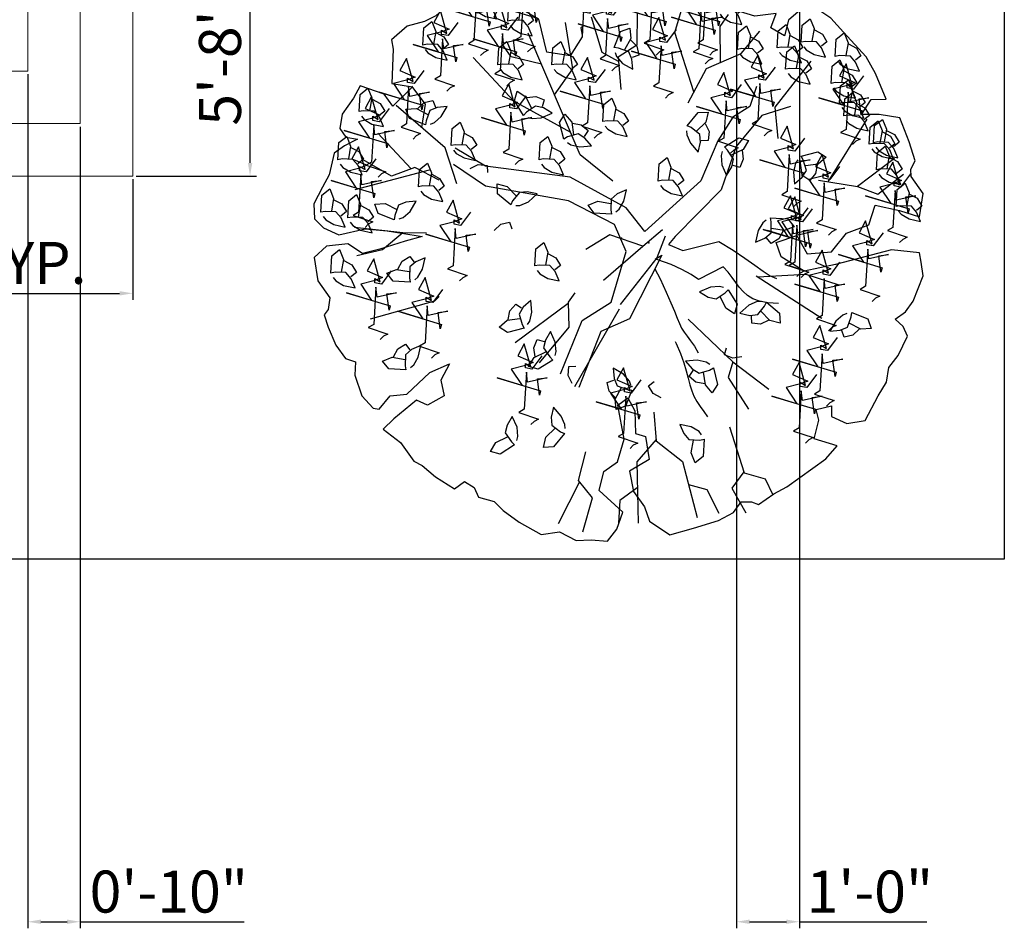
# Model space of a CAD drawing. Units: inches. Extents: x 3394 to 4794, y 965 to 1718.
# Tile 2 of 15: x 3753 to 3941, y 987 to 1160. Entities that reach past the tile are written whole.
import ezdxf

# ---------------------------------------------------------------- set-up
doc = ezdxf.new("R2010")
doc.units = ezdxf.units.IN
for name, color, linetype, lineweight in [('A-ANNO-DIMS', 2, 'Continuous', 13), ('A-FLOR-STRS', 7, 'Continuous', 18), ('C-PROP', 7, 'Continuous', 25), ('CAY', 94, 'Continuous', 13)]:
    doc.layers.add(name, color=color, linetype=linetype, lineweight=lineweight)
doc.layers.add('ARBOL', color=74, linetype='Continuous')
doc.layers.add('TALLO', color=36, linetype='Continuous')
doc.styles.get("Standard").update_dxf_attribs({"font": 'arial.ttf'})
doc.dimstyles.new('ISO-25', dxfattribs={"dimtxt": 8, "dimasz": 2.5, "dimexe": 1.25, "dimexo": 0.625, "dimtad": 1, "dimlunit": 3, "dimtxsty": 'Standard', "dimcen": 2.5, "dimadec": 0, "dimazin": 0, "dimtfac": 1, "dimtmove": 0, "dimatfit": 3, "dimfxl": 1, "dimarcsym": 0})

# ---------------------------------------------------------------- blocks, each defined once
blk = doc.blocks.new('fresno')
at = {"layer": 'ARBOL'}
for p, q in [((2.96, 0.991), (3.575, 1.984)), ((-3.638, 1.194), (-4.164, 1.76)), ((-1.151, -0.932), (-1.99, -1.556)), ((-0.974, -3.757), (-1.31, -4.423))]:
    blk.add_line(p, q, dxfattribs=at)
blk.add_lwpolyline([(0.823, 4.745), (0.566, 4.764), (0.459, 4.687), (0.336, 4.518), (0.233, 4.322), (0.087, 4.298), (0.091, 4.464), (0.14, 4.621), (-0.09, 4.659), (-0.033, 4.863), (-0.264, 4.901), (-0.483, 4.866), (-0.686, 4.924), (-1.021, 4.801), (-1.288, 4.8), (-1.431, 4.563), (-1.234, 4.327), (-1.406, 4), (-1.205, 3.778), (-0.909, 3.705), (-0.931, 3.283), (-1.122, 2.983), (-1.491, 3.043), (-1.619, 3.562), (-1.9, 3.727), (-1.851, 3.982), (-2.197, 4.084), (-2.278, 4.31), (-2.543, 4.283), (-2.896, 4.152), (-3.091, 3.971), (-3.022, 3.817), (-3.244, 3.617), (-3.424, 3.528), (-3.697, 3.455), (-3.946, 3.236), (-3.922, 3.09), (-3.94, 2.548), (-3.617, 2.495), (-3.927, 2.19), (-4.062, 2.379), (-4.443, 2.512), (-4.546, 2.316), (-4.73, 2.062), (-4.767, 1.832), (-4.671, 1.698), (-4.486, 1.667), (-4.693, 1.559), (-4.854, 1.444), (-4.934, 1.102), (-5.037, 0.905), (-5.175, 0.644), (-5.166, 0.406), (-5.024, 0.264), (-4.781, 0.153), (-4.363, 0.249), (-4.014, 0.215), (-3.783, 0.177), (-3.46, 0.124), (-3.733, 0.051), (-4.132, -0.073), (-4.404, -0.146), (-4.639, 0.011), (-4.977, -0.028), (-5.172, -0.209), (-5.113, -0.574), (-4.921, -0.843), (-4.951, -1.027), (-5.012, -1.112), (-4.95, -1.311), (-4.83, -1.592), (-4.676, -1.807), (-4.518, -1.856), (-4.529, -2.068), (-4.417, -2.394), (-4.236, -2.59), (-4.143, -2.605), (-3.967, -2.397), (-3.703, -2.37), (-3.339, -2.027), (-3.032, -1.889), (-3.169, -2.15), (-3.115, -2.396), (-3.376, -2.542), (-3.552, -2.466), (-3.909, -2.762), (-4.077, -2.924), (-3.804, -3.135), (-3.592, -3.43), (-3.461, -3.499), (-3.253, -3.676), (-2.953, -3.867), (-2.792, -3.752), (-2.642, -3.848), (-2.572, -4.001), (-2.323, -4.066), (-2.18, -4.208), (-1.926, -4.392), (-1.58, -4.591), (-1.288, -4.545), (-1.027, -4.683), (-0.788, -4.675), (-0.531, -4.693), (-0.382, -4.505), (-0.29, -4.236), (-0.66, -3.891), (-0.588, -3.595), (-0.374, -3.441), (-0.267, -3.079), (-0.368, -2.541), (-0.208, -2.426), (-0.099, -2.633), (-0.087, -2.991), (0.071, -3.04), (0.129, -3.405), (-0.185, -3.59), (-0.119, -3.909), (0.055, -4.151), (0.136, -4.377), (0.456, -4.596), (0.828, -4.491), (1.227, -4.368), (1.461, -4.241), (1.583, -4.071), (1.748, -4.075), (1.86, -4.117), (2.101, -3.944), (2.308, -3.836), (2.925, -3.393), (3.101, -3.185), (2.74, -3.078), (2.812, -2.782), (2.769, -2.61), (3.015, -2.555), (3.012, -2.721), (3.254, -2.832), (3.546, -2.785), (3.752, -2.393), (3.882, -2.177), (3.92, -1.947), (4.069, -1.758), (4.214, -1.451), (4.144, -1.297), (4.021, -1.182), (4.182, -1.067), (4.304, -0.897), (4.464, -0.497), (4.429, -0.279), (4.406, -0.133), (3.964, -0.083), (3.074, -0.315), (2.582, -0.424), (2.217, -0.197), (2.136, 0.029), (2.462, 0.141), (2.628, -0.147), (3.012, -0.116), (3.249, 0.177), (3.602, 0.308), (3.701, 0.623), (4.089, 0.535), (4.404, 0.436), (4.464, 0.805), (4.272, 1.074), (4.267, 1.193), (4.336, 1.324), (4.243, 1.623), (4.092, 2.003), (3.769, 2.057), (3.485, 2.056), (3.642, 2.291), (3.88, 2.299), (3.71, 2.706), (3.563, 2.967), (3.201, 3.358), (3.001, 3.581), (2.766, 3.738), (2.635, 3.807), (2.332, 3.549), (2.268, 3.299), (2.052, 3.429), (2.136, 3.652), (1.798, 3.613), (1.437, 3.72), (1.755, 4.071), (1.513, 4.182), (1.451, 4.381), (1.519, 4.512), (1.204, 4.611), (1.012, 4.596)], close=True, dxfattribs=at)
for points in [[(-1.104, 4.45), (-1.063, 4.399), (-0.939, 4.325), (-0.757, 4.285), (-0.82, 4.431), (-0.903, 4.527), (-1.075, 4.533), (-1.143, 4.521), (-1.126, 4.792), (-1.002, 4.891), (-0.939, 4.738), (-0.975, 4.535)], [(-0.346, 4.735), (-0.501, 4.528), (-0.605, 4.545), (-0.605, 4.614), (-0.519, 4.563), (-0.622, 4.925), (-0.726, 4.735), (-0.484, 4.632), (-0.622, 4.58), (-0.829, 4.528), (-0.657, 4.27), (-1.053, 4.39), (-0.363, 4.183), (-0.381, 4.114), (-0.415, 4.373), (-0.26, 4.39), (-0.57, 4.321), (-0.588, 4.476), (-0.622, 3.89), (-0.708, 3.839), (-0.398, 3.735), (-0.467, 3.701), (-0.519, 3.649)], [(-0.935, 4.717), (-0.809, 4.65), (-0.736, 4.529), (-0.824, 4.459)], [(0.263, 4.114), (0.304, 4.063), (0.429, 3.989), (0.611, 3.948), (0.547, 4.095), (0.465, 4.191), (0.293, 4.197), (0.225, 4.185), (0.242, 4.456), (0.366, 4.555), (0.428, 4.402), (0.393, 4.199)], [(0.734, 4.203), (0.775, 4.152), (0.9, 4.078), (1.082, 4.038), (1.018, 4.185), (0.936, 4.281), (0.763, 4.287), (0.696, 4.274), (0.712, 4.546), (0.837, 4.645), (0.899, 4.491), (0.863, 4.289)], [(-0.521, 4.069), (-0.48, 4.018), (-0.356, 3.944), (-0.174, 3.904), (-0.237, 4.051), (-0.32, 4.146), (-0.492, 4.152), (-0.56, 4.14), (-0.543, 4.411), (-0.419, 4.511), (-0.356, 4.357), (-0.392, 4.154)], [(0.433, 4.381), (0.558, 4.314), (0.631, 4.193), (0.544, 4.122)], [(0.904, 4.471), (1.029, 4.404), (1.102, 4.282), (1.015, 4.212)], [(-2.368, 4.073), (-2.523, 3.866), (-2.627, 3.883), (-2.627, 3.952), (-2.541, 3.9), (-2.644, 4.262), (-2.748, 4.073), (-2.506, 3.969), (-2.644, 3.918), (-2.851, 3.866), (-2.679, 3.607), (-3.075, 3.728), (-2.385, 3.521), (-2.403, 3.452), (-2.437, 3.711), (-2.282, 3.728), (-2.592, 3.659), (-2.61, 3.814), (-2.644, 3.228), (-2.73, 3.176), (-2.42, 3.073), (-2.489, 3.038), (-2.541, 2.987)], [(-1.623, 4.132), (-1.778, 3.925), (-1.882, 3.942), (-1.882, 4.011), (-1.795, 3.959), (-1.899, 4.321), (-2.002, 4.132), (-1.761, 4.028), (-1.899, 3.977), (-2.106, 3.925), (-1.933, 3.666), (-2.33, 3.787), (-1.64, 3.58), (-1.657, 3.511), (-1.692, 3.77), (-1.537, 3.787), (-1.847, 3.718), (-1.864, 3.873), (-1.899, 3.287), (-1.985, 3.235), (-1.675, 3.132), (-1.744, 3.097), (-1.795, 3.046)], [(-1.149, 3.822), (-1.108, 3.771), (-0.983, 3.697), (-0.802, 3.657), (-0.865, 3.804), (-0.948, 3.9), (-1.12, 3.906), (-1.188, 3.893), (-1.171, 4.165), (-1.047, 4.264), (-0.984, 4.111), (-1.02, 3.908)], [(-0.352, 4.337), (-0.226, 4.269), (-0.153, 4.148), (-0.241, 4.078)], [(0.413, 4.08), (0.258, 3.873), (0.154, 3.89), (0.154, 3.959), (0.241, 3.908), (0.137, 4.27), (0.034, 4.08), (0.275, 3.977), (0.137, 3.925), (-0.07, 3.873), (0.103, 3.614), (-0.294, 3.735), (0.396, 3.528), (0.379, 3.459), (0.344, 3.718), (0.499, 3.735), (0.189, 3.666), (0.172, 3.821), (0.137, 3.235), (0.051, 3.183), (0.361, 3.08), (0.292, 3.046), (0.241, 2.994)], [(1.259, 4.08), (1.103, 3.873), (1, 3.89), (1, 3.959), (1.086, 3.908), (0.982, 4.27), (0.879, 4.08), (1.12, 3.977), (0.982, 3.925), (0.775, 3.873), (0.948, 3.614), (0.551, 3.735), (1.241, 3.528), (1.224, 3.459), (1.189, 3.718), (1.345, 3.735), (1.034, 3.666), (1.017, 3.821), (0.982, 3.235), (0.896, 3.183), (1.207, 3.08), (1.138, 3.046), (1.086, 2.994)], [(-2.629, 3.733), (-2.588, 3.682), (-2.463, 3.608), (-2.281, 3.568), (-2.345, 3.715), (-2.427, 3.81), (-2.6, 3.816), (-2.667, 3.804), (-2.651, 4.075), (-2.526, 4.175), (-2.464, 4.021), (-2.5, 3.818)], [(-0.98, 4.09), (-0.854, 4.023), (-0.781, 3.901), (-0.869, 3.831)], [(1.189, 3.942), (1.034, 3.735), (0.931, 3.752), (0.931, 3.821), (1.017, 3.77), (0.913, 4.132), (0.81, 3.942), (1.051, 3.839), (0.913, 3.787), (0.706, 3.735), (0.879, 3.477), (0.482, 3.597), (1.172, 3.39), (1.155, 3.321), (1.12, 3.58), (1.276, 3.597), (0.965, 3.528), (0.948, 3.683), (0.913, 3.097), (0.827, 3.046), (1.138, 2.942), (1.069, 2.908), (1.017, 2.856)], [(1.25, 3.643), (1.291, 3.592), (1.416, 3.518), (1.597, 3.478), (1.534, 3.625), (1.451, 3.721), (1.279, 3.727), (1.211, 3.714), (1.228, 3.985), (1.352, 4.085), (1.415, 3.931), (1.379, 3.729)], [(-2.459, 4), (-2.334, 3.933), (-2.261, 3.812), (-2.348, 3.742)], [(-2.068, 3.464), (-2.027, 3.413), (-1.903, 3.339), (-1.721, 3.299), (-1.784, 3.446), (-1.867, 3.542), (-2.039, 3.547), (-2.107, 3.535), (-2.09, 3.806), (-1.966, 3.906), (-1.903, 3.752), (-1.939, 3.55)], [(-0.287, 3.833), (-0.442, 3.626), (-0.546, 3.643), (-0.546, 3.712), (-0.46, 3.661), (-0.563, 4.023), (-0.667, 3.833), (-0.425, 3.73), (-0.563, 3.678), (-0.77, 3.626), (-0.598, 3.367), (-0.995, 3.488), (-0.304, 3.281), (-0.322, 3.212), (-0.356, 3.471), (-0.201, 3.488), (-0.511, 3.419), (-0.529, 3.574), (-0.563, 2.988), (-0.649, 2.936), (-0.339, 2.833), (-0.408, 2.799), (-0.46, 2.747)], [(0.837, 2.414), (0.533, 3.352), (0.697, 3.906)], [(1.419, 3.911), (1.545, 3.844), (1.618, 3.722), (1.53, 3.652)], [(-1.951, 3.597), (-2.106, 3.39), (-2.209, 3.408), (-2.209, 3.477), (-2.123, 3.425), (-2.227, 3.787), (-2.33, 3.597), (-2.089, 3.494), (-2.227, 3.442), (-2.434, 3.39), (-2.261, 3.132), (-2.658, 3.252), (-1.968, 3.046), (-1.985, 2.977), (-2.02, 3.235), (-1.864, 3.252), (-2.175, 3.183), (-2.192, 3.339), (-2.227, 2.752), (-2.313, 2.701), (-2.002, 2.597), (-2.071, 2.563), (-2.123, 2.511)], [(-2.898, 3.511), (-3.053, 3.304), (-3.157, 3.321), (-3.157, 3.39), (-3.071, 3.339), (-3.174, 3.701), (-3.278, 3.511), (-3.036, 3.408), (-3.174, 3.356), (-3.381, 3.304), (-3.209, 3.046), (-3.605, 3.166), (-2.915, 2.959), (-2.932, 2.89), (-2.967, 3.149), (-2.812, 3.166), (-3.122, 3.097), (-3.14, 3.253), (-3.174, 2.666), (-3.26, 2.615), (-2.95, 2.511), (-3.019, 2.477), (-3.071, 2.425)], [(-1.899, 3.732), (-1.773, 3.664), (-1.7, 3.543), (-1.788, 3.473)], [(-0.358, 2.895), (-0.615, 3.037), (-0.783, 3.596)], [(-0.063, 3.671), (-0.069, 3.151), (-0.364, 2.965), (-0.319, 2.449)], [(0.558, 3.402), (0.403, 3.195), (0.299, 3.212), (0.299, 3.281), (0.386, 3.23), (0.282, 3.592), (0.179, 3.402), (0.42, 3.299), (0.282, 3.247), (0.075, 3.195), (0.248, 2.936), (-0.149, 3.057), (0.541, 2.85), (0.524, 2.781), (0.489, 3.04), (0.644, 3.057), (0.334, 2.988), (0.317, 3.143), (0.282, 2.557), (0.196, 2.505), (0.506, 2.402), (0.437, 2.368), (0.386, 2.316)], [(1.259, 2.882), (1.254, 3.446), (1.381, 3.636)], [(-3.413, 3.083), (-3.373, 3.032), (-3.248, 2.958), (-3.066, 2.918), (-3.129, 3.065), (-3.212, 3.161), (-3.384, 3.167), (-3.452, 3.154), (-3.435, 3.425), (-3.311, 3.525), (-3.248, 3.371), (-3.284, 3.169)], [(-1.367, 2.367), (-1.081, 2.78), (-1.193, 3.514)], [(-0.923, 3.449), (-0.951, 3.425), (-0.93, 3.313)], [(1.564, 3.016), (1.605, 2.965), (1.729, 2.891), (1.911, 2.851), (1.848, 2.998), (1.765, 3.094), (1.593, 3.099), (1.525, 3.087), (1.542, 3.358), (1.666, 3.458), (1.729, 3.304), (1.693, 3.102)], [(2.191, 3.038), (2.232, 2.987), (2.357, 2.913), (2.539, 2.873), (2.475, 3.02), (2.393, 3.116), (2.221, 3.122), (2.153, 3.109), (2.17, 3.381), (2.294, 3.48), (2.356, 3.326), (2.321, 3.124)], [(2.573, 3.128), (2.613, 3.077), (2.738, 3.003), (2.92, 2.963), (2.857, 3.11), (2.774, 3.205), (2.602, 3.211), (2.534, 3.199), (2.551, 3.47), (2.675, 3.57), (2.738, 3.416), (2.702, 3.214)], [(-3.244, 3.351), (-3.118, 3.284), (-3.045, 3.162), (-3.133, 3.092)], [(-0.448, 1), (-0.961, 1.419), (-1.784, 3.341)], [(-0.41, 3.035), (-0.387, 2.974), (-0.291, 2.865), (-0.131, 2.771), (-0.146, 2.93), (-0.195, 3.047), (-0.357, 3.106), (-0.425, 3.115), (-0.325, 3.368), (-0.176, 3.424), (-0.164, 3.258), (-0.261, 3.077)], [(0.746, 2.242), (1.034, 2.786), (1.584, 3.019), (1.879, 3.374)], [(1.733, 3.284), (1.859, 3.216), (1.932, 3.095), (1.844, 3.025)], [(2.361, 3.306), (2.486, 3.239), (2.559, 3.117), (2.472, 3.047)], [(2.742, 3.396), (2.868, 3.328), (2.941, 3.207), (2.853, 3.137)], [(3.111, 2.904), (3.152, 2.853), (3.276, 2.779), (3.458, 2.739), (3.395, 2.886), (3.312, 2.981), (3.14, 2.987), (3.072, 2.975), (3.089, 3.246), (3.213, 3.346), (3.276, 3.192), (3.24, 2.99)], [(-2.225, 2.77), (-2.184, 2.718), (-2.06, 2.645), (-1.878, 2.604), (-1.941, 2.751), (-2.024, 2.847), (-2.196, 2.853), (-2.264, 2.84), (-2.247, 3.112), (-2.123, 3.211), (-2.06, 3.058), (-2.096, 2.855)], [(-1.575, 2.854), (-2.052, 2.969), (-2.2, 3.178)], [(-1.373, 2.77), (-1.332, 2.718), (-1.208, 2.645), (-1.026, 2.604), (-1.089, 2.751), (-1.172, 2.847), (-1.344, 2.853), (-1.412, 2.84), (-1.395, 3.112), (-1.271, 3.211), (-1.208, 3.058), (-1.244, 2.855)], [(-0.166, 3.238), (-0.068, 3.135), (-0.036, 2.997), (-0.141, 2.957)], [(2.326, 2.702), (2.367, 2.651), (2.492, 2.577), (2.673, 2.537), (2.61, 2.684), (2.527, 2.78), (2.355, 2.786), (2.287, 2.773), (2.304, 3.045), (2.428, 3.144), (2.491, 2.99), (2.455, 2.788)], [(3.28, 3.172), (3.406, 3.104), (3.479, 2.983), (3.391, 2.913)], [(-2.056, 3.037), (-1.93, 2.97), (-1.857, 2.849), (-1.945, 2.778)], [(-0.57, 2.77), (-0.726, 2.563), (-0.829, 2.58), (-0.829, 2.649), (-0.743, 2.597), (-0.846, 2.959), (-0.95, 2.77), (-0.708, 2.666), (-0.846, 2.615), (-1.053, 2.563), (-0.881, 2.304), (-1.278, 2.425), (-0.588, 2.218), (-0.605, 2.149), (-0.639, 2.408), (-0.484, 2.425), (-0.795, 2.356), (-0.812, 2.511), (-0.846, 1.925), (-0.933, 1.873), (-0.622, 1.77), (-0.691, 1.735), (-0.743, 1.684)], [(-1.204, 3.037), (-1.078, 2.97), (-1.005, 2.849), (-1.093, 2.778)], [(2.121, 2.804), (1.966, 2.597), (1.862, 2.615), (1.862, 2.683), (1.949, 2.632), (1.845, 2.994), (1.742, 2.804), (1.983, 2.701), (1.845, 2.649), (1.638, 2.597), (1.811, 2.339), (1.414, 2.459), (2.104, 2.252), (2.087, 2.184), (2.052, 2.442), (2.207, 2.459), (1.897, 2.39), (1.88, 2.546), (1.845, 1.959), (1.759, 1.908), (2.069, 1.804), (2, 1.77), (1.949, 1.718)], [(2.495, 2.97), (2.621, 2.903), (2.694, 2.781), (2.606, 2.711)], [(-3.434, 2.752), (-3.59, 2.546), (-3.693, 2.563), (-3.693, 2.632), (-3.607, 2.58), (-3.71, 2.942), (-3.814, 2.752), (-3.572, 2.649), (-3.71, 2.597), (-3.917, 2.546), (-3.745, 2.287), (-4.142, 2.408), (-3.452, 2.201), (-3.469, 2.132), (-3.503, 2.39), (-3.348, 2.408), (-3.659, 2.339), (-3.676, 2.494), (-3.71, 1.908), (-3.797, 1.856), (-3.486, 1.753), (-3.555, 1.718), (-3.607, 1.666)], [(-1.112, 1.773), (-2.014, 2.265), (-2.654, 2.957)], [(2.171, 1.674), (2.121, 2.172), (2.689, 2.898)], [(3.519, 2.666), (3.363, 2.459), (3.26, 2.477), (3.26, 2.546), (3.346, 2.494), (3.243, 2.856), (3.139, 2.666), (3.381, 2.563), (3.243, 2.511), (3.036, 2.459), (3.208, 2.201), (2.811, 2.321), (3.501, 2.115), (3.484, 2.046), (3.45, 2.304), (3.605, 2.321), (3.294, 2.252), (3.277, 2.408), (3.243, 1.821), (3.156, 1.77), (3.467, 1.666), (3.398, 1.632), (3.346, 1.58)], [(3.043, 2.478), (3.084, 2.427), (3.209, 2.353), (3.391, 2.313), (3.327, 2.46), (3.245, 2.556), (3.073, 2.562), (3.005, 2.549), (3.022, 2.82), (3.146, 2.92), (3.208, 2.766), (3.173, 2.564)], [(1.586, 2.528), (1.431, 2.321), (1.327, 2.339), (1.327, 2.408), (1.414, 2.356), (1.31, 2.718), (1.207, 2.528), (1.448, 2.425), (1.31, 2.373), (1.103, 2.321), (1.276, 2.063), (0.879, 2.184), (1.569, 1.977), (1.552, 1.908), (1.517, 2.166), (1.673, 2.184), (1.362, 2.115), (1.345, 2.27), (1.31, 1.684), (1.224, 1.632), (1.535, 1.528), (1.466, 1.494), (1.414, 1.442)], [(3.213, 2.746), (3.338, 2.679), (3.411, 2.557), (3.324, 2.487)], [(-3.468, 1.85), (-3.409, 2.222), (-3.628, 2.505)], [(-1.817, 2.351), (-1.972, 2.144), (-2.075, 2.162), (-2.075, 2.231), (-1.989, 2.179), (-2.093, 2.541), (-2.196, 2.351), (-1.955, 2.248), (-2.093, 2.196), (-2.3, 2.144), (-2.127, 1.886), (-2.524, 2.006), (-1.834, 1.8), (-1.851, 1.731), (-1.886, 1.989), (-1.73, 2.006), (-2.041, 1.937), (-2.058, 2.093), (-2.093, 1.506), (-2.179, 1.455), (-1.868, 1.351), (-1.937, 1.317), (-1.989, 1.265)], [(3.178, 2.165), (3.219, 2.113), (3.344, 2.04), (3.525, 1.999), (3.462, 2.146), (3.379, 2.242), (3.207, 2.248), (3.139, 2.236), (3.156, 2.507), (3.28, 2.606), (3.343, 2.453), (3.307, 2.25)], [(-3.986, 2.149), (-4.142, 1.942), (-4.245, 1.959), (-4.245, 2.028), (-4.159, 1.977), (-4.262, 2.339), (-4.366, 2.149), (-4.124, 2.046), (-4.262, 1.994), (-4.47, 1.942), (-4.297, 1.684), (-4.694, 1.804), (-4.004, 1.597), (-4.021, 1.528), (-4.055, 1.787), (-3.9, 1.804), (-4.211, 1.735), (-4.228, 1.89), (-4.262, 1.304), (-4.349, 1.253), (-4.038, 1.149), (-4.107, 1.115), (-4.159, 1.063)], [(-4.422, 2.03), (-4.381, 1.979), (-4.257, 1.905), (-4.075, 1.865), (-4.138, 2.012), (-4.221, 2.108), (-4.393, 2.114), (-4.461, 2.101), (-4.444, 2.372), (-4.32, 2.472), (-4.257, 2.318), (-4.293, 2.116)], [(-1.786, 2.007), (-1.722, 1.99), (-1.578, 2.003), (-1.407, 2.078), (-1.545, 2.159), (-1.668, 2.188), (-1.811, 2.092), (-1.859, 2.042), (-2.004, 2.271), (-1.962, 2.425), (-1.821, 2.337), (-1.731, 2.152)], [(-1.806, 2.323), (-1.665, 2.343), (-1.534, 2.287), (-1.564, 2.179)], [(3.245, 1.963), (3.286, 1.912), (3.411, 1.838), (3.593, 1.798), (3.529, 1.945), (3.447, 2.041), (3.274, 2.046), (3.206, 2.034), (3.223, 2.305), (3.347, 2.405), (3.41, 2.251), (3.374, 2.049)], [(3.347, 2.432), (3.473, 2.365), (3.546, 2.244), (3.458, 2.173)], [(-4.253, 2.298), (-4.127, 2.231), (-4.054, 2.109), (-4.142, 2.039)], [(-2.916, 0.958), (-3.096, 1.528), (-3.871, 2.197)], [(-3.331, 1.905), (-3.269, 1.928), (-3.161, 2.024), (-3.066, 2.184), (-3.226, 2.169), (-3.342, 2.121), (-3.401, 1.958), (-3.41, 1.89), (-3.663, 1.99), (-3.719, 2.139), (-3.554, 2.151), (-3.372, 2.054)], [(-3.533, 2.149), (-3.43, 2.247), (-3.292, 2.279), (-3.252, 2.174)], [(-0.566, 1.873), (-0.525, 1.822), (-0.4, 1.748), (-0.219, 1.708), (-0.282, 1.855), (-0.365, 1.951), (-0.537, 1.957), (-0.605, 1.944), (-0.588, 2.216), (-0.464, 2.315), (-0.401, 2.162), (-0.437, 1.959)], [(3.415, 2.231), (3.54, 2.163), (3.613, 2.042), (3.525, 1.972)], [(-1.164, 1.612), (-1.109, 1.576), (-0.967, 1.544), (-0.782, 1.562), (-0.888, 1.682), (-0.996, 1.748), (-1.162, 1.7), (-1.222, 1.667), (-1.29, 1.93), (-1.203, 2.063), (-1.096, 1.937), (-1.067, 1.733)], [(-0.397, 2.141), (-0.271, 2.074), (-0.198, 1.952), (-0.286, 1.882)], [(0.72, 1.798), (0.723, 1.733), (0.781, 1.6), (0.904, 1.46), (0.939, 1.616), (0.929, 1.742), (0.793, 1.848), (0.73, 1.878), (0.904, 2.088), (1.062, 2.095), (1.023, 1.934), (0.875, 1.791)], [(-2.965, 1.493), (-2.924, 1.441), (-2.799, 1.368), (-2.618, 1.327), (-2.681, 1.474), (-2.764, 1.57), (-2.936, 1.576), (-3.004, 1.564), (-2.987, 1.835), (-2.863, 1.934), (-2.8, 1.781), (-2.836, 1.578)], [(-1.085, 1.919), (-0.945, 1.893), (-0.838, 1.801), (-0.9, 1.707)], [(1.014, 1.915), (1.077, 1.787), (1.064, 1.646), (0.952, 1.64)], [(2.587, 1.684), (2.432, 1.477), (2.328, 1.494), (2.328, 1.563), (2.414, 1.511), (2.311, 1.873), (2.207, 1.684), (2.449, 1.58), (2.311, 1.528), (2.104, 1.477), (2.276, 1.218), (1.88, 1.339), (2.57, 1.132), (2.552, 1.063), (2.518, 1.321), (2.673, 1.339), (2.363, 1.27), (2.345, 1.425), (2.311, 0.839), (2.225, 0.787), (2.535, 0.684), (2.466, 0.649), (2.414, 0.597)], [(3.649, 1.515), (3.69, 1.464), (3.814, 1.39), (3.996, 1.35), (3.933, 1.497), (3.85, 1.592), (3.678, 1.598), (3.61, 1.586), (3.627, 1.857), (3.751, 1.957), (3.814, 1.803), (3.778, 1.601)], [(3.716, 1.537), (3.757, 1.486), (3.882, 1.412), (4.063, 1.372), (4, 1.519), (3.917, 1.615), (3.745, 1.621), (3.677, 1.608), (3.694, 1.88), (3.818, 1.979), (3.881, 1.825), (3.845, 1.623)], [(-2.796, 1.76), (-2.67, 1.693), (-2.597, 1.572), (-2.685, 1.501)], [(3.818, 1.783), (3.944, 1.715), (4.017, 1.594), (3.929, 1.524)], [(3.885, 1.805), (4.011, 1.738), (4.084, 1.616), (3.996, 1.546)], [(-4.759, 1.269), (-4.718, 1.217), (-4.593, 1.144), (-4.411, 1.103), (-4.475, 1.25), (-4.557, 1.346), (-4.729, 1.352), (-4.797, 1.339), (-4.78, 1.611), (-4.656, 1.71), (-4.594, 1.557), (-4.629, 1.354)], [(-1.575, 1.269), (-1.534, 1.217), (-1.409, 1.144), (-1.228, 1.103), (-1.291, 1.25), (-1.373, 1.346), (-1.546, 1.352), (-1.614, 1.339), (-1.597, 1.611), (-1.473, 1.71), (-1.41, 1.557), (-1.446, 1.354)], [(1.283, 1.469), (1.266, 1.405), (1.279, 1.261), (1.354, 1.09), (1.435, 1.228), (1.464, 1.351), (1.368, 1.494), (1.318, 1.542), (1.547, 1.687), (1.7, 1.645), (1.613, 1.504), (1.428, 1.414)], [(-4.193, 1.356), (-4.349, 1.149), (-4.452, 1.166), (-4.452, 1.235), (-4.366, 1.184), (-4.469, 1.546), (-4.573, 1.356), (-4.331, 1.253), (-4.469, 1.201), (-4.677, 1.149), (-4.504, 0.89), (-4.901, 1.011), (-4.211, 0.804), (-4.228, 0.735), (-4.262, 0.994), (-4.107, 1.011), (-4.418, 0.942), (-4.435, 1.097), (-4.469, 0.511), (-4.556, 0.459), (-4.245, 0.356), (-4.314, 0.322), (-4.366, 0.27)], [(-4.589, 1.536), (-4.464, 1.469), (-4.391, 1.348), (-4.478, 1.277)], [(-1.406, 1.536), (-1.28, 1.469), (-1.207, 1.348), (-1.295, 1.277)], [(1.599, 1.489), (1.618, 1.348), (1.563, 1.217), (1.455, 1.247)], [(2.479, 1.34), (2.443, 1.285), (2.411, 1.143), (2.429, 0.958), (2.549, 1.064), (2.615, 1.172), (2.567, 1.338), (2.534, 1.398), (2.797, 1.466), (2.93, 1.379), (2.804, 1.272), (2.6, 1.243)], [(3.139, 1.235), (2.984, 1.028), (2.88, 1.046), (2.88, 1.115), (2.967, 1.063), (2.863, 1.425), (2.759, 1.235), (3.001, 1.132), (2.863, 1.08), (2.656, 1.028), (2.828, 0.77), (2.432, 0.891), (3.122, 0.684), (3.105, 0.615), (3.07, 0.873), (3.225, 0.891), (2.915, 0.822), (2.897, 0.977), (2.863, 0.391), (2.777, 0.339), (3.087, 0.235), (3.018, 0.201), (2.967, 0.149)], [(3.761, 1.112), (3.802, 1.061), (3.926, 0.987), (4.108, 0.947), (4.045, 1.093), (3.962, 1.189), (3.79, 1.195), (3.722, 1.183), (3.739, 1.454), (3.863, 1.553), (3.926, 1.4), (3.89, 1.197)], [(-3.192, 1.017), (-3.578, 1.215), (-3.949, 1.081), (-4.398, 1.339)], [(-3.481, 0.843), (-3.44, 0.792), (-3.315, 0.718), (-3.133, 0.678), (-3.197, 0.825), (-3.279, 0.92), (-3.451, 0.926), (-3.519, 0.914), (-3.502, 1.185), (-3.378, 1.285), (-3.316, 1.131), (-3.351, 0.928)], [(-2.703, 1.201), (-2.575, 1.263), (-2.433, 1.251), (-2.428, 1.139)], [(0.308, 0.933), (0.349, 0.881), (0.474, 0.807), (0.656, 0.767), (0.592, 0.914), (0.51, 1.01), (0.337, 1.016), (0.27, 1.003), (0.286, 1.275), (0.411, 1.374), (0.473, 1.221), (0.437, 1.018)], [(2.786, 1.261), (2.76, 1.121), (2.668, 1.014), (2.574, 1.076)], [(4.01, 1.36), (3.422, 0.918)], [(4.26, 1.115), (4.105, 0.908), (4.002, 0.925), (4.002, 0.994), (4.088, 0.942), (3.984, 1.304), (3.881, 1.115), (4.122, 1.011), (3.984, 0.959), (3.777, 0.908), (3.95, 0.649), (3.553, 0.77), (4.243, 0.563), (4.226, 0.494), (4.191, 0.753), (4.347, 0.77), (4.036, 0.701), (4.019, 0.856), (3.984, 0.27), (3.898, 0.218), (4.209, 0.115), (4.14, 0.08), (4.088, 0.029)], [(3.93, 1.379), (4.056, 1.312), (4.129, 1.191), (4.041, 1.121)], [(-3.354, 1.176), (-4.529, 0.864)], [(-3.311, 1.111), (-3.186, 1.043), (-3.113, 0.922), (-3.2, 0.852)], [(0.478, 1.2), (0.603, 1.133), (0.676, 1.011), (0.589, 0.941)], [(2.808, 1.015), (3.422, 0.918), (3.422, 0.918), (3.748, 0.794), (4.154, 1.111)], [(-1.981, 0.615), (-1.915, 0.618), (-1.782, 0.676), (-1.643, 0.799), (-1.799, 0.834), (-1.925, 0.824), (-2.031, 0.688), (-2.061, 0.626), (-2.27, 0.799), (-2.278, 0.958), (-2.117, 0.918), (-1.974, 0.77)], [(4.075, 0.529), (4.116, 0.478), (4.24, 0.404), (4.422, 0.364), (4.359, 0.511), (4.276, 0.607), (4.104, 0.613), (4.036, 0.6), (4.053, 0.871), (4.177, 0.971), (4.24, 0.817), (4.204, 0.615)], [(-5.028, 0.44), (-4.987, 0.388), (-4.862, 0.315), (-4.68, 0.274), (-4.744, 0.421), (-4.826, 0.517), (-4.998, 0.523), (-5.066, 0.511), (-5.049, 0.782), (-4.925, 0.881), (-4.863, 0.728), (-4.898, 0.525)], [(-4.602, 0.35), (-4.561, 0.299), (-4.436, 0.225), (-4.254, 0.185), (-4.318, 0.332), (-4.4, 0.428), (-4.572, 0.433), (-4.64, 0.421), (-4.623, 0.692), (-4.499, 0.792), (-4.437, 0.638), (-4.472, 0.436)], [(-0.397, 0.517), (-0.346, 0.557), (-0.272, 0.682), (-0.232, 0.864), (-0.379, 0.801), (-0.474, 0.718), (-0.48, 0.546), (-0.468, 0.478), (-0.739, 0.495), (-0.838, 0.619), (-0.685, 0.682), (-0.482, 0.646)], [(4.244, 0.797), (4.37, 0.73), (4.443, 0.608), (4.355, 0.538)], [(-4.858, 0.707), (-4.733, 0.64), (-4.66, 0.519), (-4.747, 0.448)], [(-3.824, 0.404), (-3.763, 0.427), (-3.654, 0.523), (-3.559, 0.683), (-3.719, 0.668), (-3.835, 0.62), (-3.894, 0.457), (-3.903, 0.389), (-4.156, 0.489), (-4.212, 0.638), (-4.047, 0.65), (-3.865, 0.553)], [(-2.698, 0.509), (-2.854, 0.302), (-2.957, 0.319), (-2.957, 0.388), (-2.871, 0.336), (-2.974, 0.698), (-3.078, 0.509), (-2.836, 0.405), (-2.974, 0.353), (-3.182, 0.302), (-3.009, 0.043), (-3.406, 0.164), (-2.716, -0.043), (-2.733, -0.112), (-2.767, 0.147), (-2.612, 0.164), (-2.923, 0.095), (-2.94, 0.25), (-2.974, -0.336), (-3.061, -0.388), (-2.75, -0.491), (-2.819, -0.526), (-2.871, -0.577)], [(2.639, 0.58), (2.483, 0.373), (2.38, 0.391), (2.38, 0.46), (2.466, 0.408), (2.363, 0.77), (2.259, 0.58), (2.501, 0.477), (2.363, 0.425), (2.156, 0.373), (2.328, 0.115), (1.931, 0.235), (2.621, 0.029), (2.604, -0.04), (2.57, 0.218), (2.725, 0.235), (2.414, 0.166), (2.397, 0.322), (2.363, -0.265), (2.276, -0.316), (2.587, -0.42), (2.518, -0.454), (2.466, -0.506)], [(2.708, 0.563), (2.552, 0.356), (2.449, 0.373), (2.449, 0.442), (2.535, 0.391), (2.432, 0.753), (2.328, 0.563), (2.57, 0.46), (2.432, 0.408), (2.225, 0.356), (2.397, 0.097), (2, 0.218), (2.69, 0.011), (2.673, -0.058), (2.639, 0.201), (2.794, 0.218), (2.483, 0.149), (2.466, 0.304), (2.432, -0.282), (2.345, -0.334), (2.656, -0.437), (2.587, -0.471), (2.535, -0.523)], [(-4.432, 0.618), (-4.307, 0.55), (-4.234, 0.429), (-4.321, 0.359)], [(-2.322, 0.222), (-2.219, 0.321), (-2.081, 0.353), (-2.042, 0.248)], [(1.978, 0.384), (1.927, 0.343), (1.853, 0.218), (1.813, 0.036), (1.96, 0.1), (2.056, 0.182), (2.061, 0.355), (2.049, 0.422), (2.32, 0.406), (2.42, 0.281), (2.266, 0.219), (2.064, 0.254)], [(3.829, 0.184), (3.674, -0.023), (3.57, -0.006), (3.57, 0.063), (3.657, 0.011), (3.553, 0.373), (3.45, 0.184), (3.691, 0.08), (3.553, 0.029), (3.346, -0.023), (3.519, -0.282), (3.122, -0.161), (3.812, -0.368), (3.795, -0.437), (3.76, -0.178), (3.915, -0.161), (3.605, -0.23), (3.588, -0.075), (3.553, -0.661), (3.467, -0.713), (3.777, -0.816), (3.708, -0.851), (3.657, -0.902)], [(-3.394, 0.18), (-3.77, 0.182), (-4.532, 0.27)], [(-3.77, 0.182), (-4.09, -0.088), (-4.494, -0.18)], [(-0.596, -0.564), (0.03, -0.026), (0.339, 0.235)], [(2.246, 0.214), (2.178, 0.089), (2.057, 0.016), (1.987, 0.103)], [(-1.642, -0.412), (-1.601, -0.463), (-1.477, -0.537), (-1.295, -0.577), (-1.358, -0.43), (-1.441, -0.334), (-1.613, -0.328), (-1.681, -0.341), (-1.664, -0.069), (-1.54, 0.03), (-1.477, -0.124), (-1.513, -0.326)], [(0.03, -0.026), (-0.491, 0.154), (-0.871, -0.08)], [(0.38, 0.131), (0.248, -0.21), (-0.33, -0.951)], [(-4.871, -0.524), (-4.83, -0.575), (-4.705, -0.649), (-4.523, -0.689), (-4.587, -0.542), (-4.669, -0.446), (-4.841, -0.44), (-4.909, -0.453), (-4.893, -0.181), (-4.768, -0.082), (-4.706, -0.236), (-4.741, -0.438)], [(-1.473, -0.144), (-1.347, -0.211), (-1.274, -0.333), (-1.362, -0.403)], [(3.139, -0.282), (2.984, -0.489), (2.88, -0.471), (2.88, -0.402), (2.967, -0.454), (2.863, -0.092), (2.759, -0.282), (3.001, -0.385), (2.863, -0.437), (2.656, -0.489), (2.828, -0.747), (2.432, -0.627), (3.122, -0.834), (3.105, -0.902), (3.07, -0.644), (3.225, -0.627), (2.915, -0.696), (2.897, -0.54), (2.863, -1.127), (2.777, -1.178), (3.087, -1.282), (3.018, -1.316), (2.967, -1.368)], [(-4.701, -0.256), (-4.576, -0.323), (-4.503, -0.445), (-4.59, -0.515)], [(-3.952, -0.42), (-4.107, -0.627), (-4.211, -0.609), (-4.211, -0.54), (-4.124, -0.592), (-4.228, -0.23), (-4.331, -0.42), (-4.09, -0.523), (-4.228, -0.575), (-4.435, -0.627), (-4.262, -0.885), (-4.659, -0.765), (-3.969, -0.971), (-3.986, -1.04), (-4.021, -0.782), (-3.866, -0.765), (-4.176, -0.834), (-4.193, -0.678), (-4.228, -1.265), (-4.314, -1.316), (-4.004, -1.42), (-4.073, -1.454), (-4.124, -1.506)], [(-3.58, -0.559), (-3.529, -0.518), (-3.455, -0.393), (-3.415, -0.211), (-3.562, -0.275), (-3.658, -0.357), (-3.664, -0.53), (-3.651, -0.597), (-3.923, -0.581), (-4.022, -0.456), (-3.868, -0.394), (-3.666, -0.43)], [(-3.848, -0.389), (-3.781, -0.264), (-3.659, -0.191), (-3.589, -0.278)], [(-3.141, -0.713), (-3.296, -0.92), (-3.4, -0.902), (-3.4, -0.834), (-3.314, -0.885), (-3.417, -0.523), (-3.521, -0.713), (-3.279, -0.816), (-3.417, -0.868), (-3.624, -0.92), (-3.452, -1.178), (-3.848, -1.058), (-3.158, -1.265), (-3.175, -1.333), (-3.21, -1.075), (-3.055, -1.058), (-3.365, -1.127), (-3.383, -0.971), (-3.417, -1.558), (-3.503, -1.609), (-3.193, -1.713), (-3.262, -1.747), (-3.314, -1.799)], [(1.822, -0.495), (2.859, -1.165)], [(1.846, -0.51), (2.605, -0.469), (3.129, -0.637)], [(-1.047, -0.767), (-1.151, -0.913), (-1.144, -1.307), (-1.61, -1.871)], [(1.304, -0.681), (1.241, -0.664), (1.097, -0.678), (0.926, -0.752), (1.064, -0.833), (1.187, -0.862), (1.33, -0.766), (1.377, -0.716), (1.523, -0.945), (1.481, -1.099), (1.34, -1.011), (1.25, -0.826)], [(-3.195, -0.824), (-3.267, -0.898), (-4.285, -1.185)], [(-1.794, -1.268), (-1.758, -1.214), (-1.726, -1.072), (-1.744, -0.887), (-1.865, -0.993), (-1.93, -1.101), (-1.883, -1.266), (-1.85, -1.327), (-2.113, -1.395), (-2.246, -1.307), (-2.119, -1.2), (-1.916, -1.172)], [(1.903, -0.903), (1.837, -0.905), (1.704, -0.963), (1.565, -1.086), (1.721, -1.122), (1.847, -1.111), (1.953, -0.975), (1.983, -0.913), (2.192, -1.086), (2.2, -1.245), (2.039, -1.205), (1.896, -1.057)], [(-2.101, -1.19), (-2.076, -1.05), (-1.983, -0.943), (-1.889, -1.004)], [(-0.346, -1.024), (-1.05, -2.251)], [(3.253, -1.094), (3.192, -1.117), (3.083, -1.213), (2.988, -1.374), (3.148, -1.359), (3.264, -1.31), (3.323, -1.148), (3.332, -1.079), (3.585, -1.179), (3.641, -1.328), (3.476, -1.34), (3.294, -1.244)], [(0.748, -1.185), (1.452, -1.855), (2.021, -2.292)], [(2.02, -1.197), (1.891, -1.259), (1.75, -1.247), (1.745, -1.134)], [(-1.361, -1.756), (-1.343, -1.693), (-1.357, -1.548), (-1.431, -1.377), (-1.513, -1.515), (-1.542, -1.638), (-1.445, -1.781), (-1.395, -1.829), (-1.625, -1.974), (-1.778, -1.932), (-1.691, -1.791), (-1.506, -1.701)], [(3.105, -1.471), (2.949, -1.678), (2.846, -1.661), (2.846, -1.592), (2.932, -1.644), (2.829, -1.282), (2.725, -1.471), (2.967, -1.575), (2.829, -1.627), (2.621, -1.678), (2.794, -1.937), (2.397, -1.816), (3.087, -2.023), (3.07, -2.092), (3.036, -1.833), (3.191, -1.816), (2.88, -1.885), (2.863, -1.73), (2.829, -2.316), (2.742, -2.368), (3.053, -2.471), (2.984, -2.506), (2.932, -2.558)], [(3.455, -1.338), (3.352, -1.437), (3.214, -1.469), (3.175, -1.364)], [(-1.677, -1.776), (-1.696, -1.635), (-1.641, -1.504), (-1.533, -1.534)], [(-3.648, -1.948), (-3.596, -1.907), (-3.523, -1.782), (-3.482, -1.6), (-3.629, -1.664), (-3.725, -1.746), (-3.731, -1.919), (-3.719, -1.986), (-3.99, -1.97), (-4.089, -1.845), (-3.936, -1.783), (-3.733, -1.819)], [(-3.915, -1.778), (-3.848, -1.653), (-3.727, -1.58), (-3.656, -1.667)], [(-1.571, -1.764), (-1.726, -1.971), (-1.83, -1.954), (-1.83, -1.885), (-1.744, -1.937), (-1.847, -1.575), (-1.951, -1.764), (-1.709, -1.868), (-1.847, -1.92), (-2.054, -1.971), (-1.882, -2.23), (-2.278, -2.109), (-1.588, -2.316), (-1.605, -2.385), (-1.64, -2.127), (-1.485, -2.109), (-1.795, -2.178), (-1.813, -2.023), (-1.847, -2.609), (-1.933, -2.661), (-1.623, -2.764), (-1.692, -2.799), (-1.744, -2.851)], [(1.593, -1.781), (1.452, -1.801), (1.322, -1.746), (1.352, -1.637)], [(1.086, -1.899), (1.031, -1.863), (0.89, -1.831), (0.704, -1.849), (0.81, -1.969), (0.918, -2.035), (1.084, -1.987), (1.145, -1.954), (1.212, -2.218), (1.125, -2.35), (1.018, -2.224), (0.989, -2.02)], [(1.452, -1.855), (1.379, -2.105), (1.698, -2.609)], [(2.777, -2.058), (2.621, -2.264), (2.518, -2.247), (2.518, -2.178), (2.604, -2.23), (2.501, -1.868), (2.397, -2.058), (2.639, -2.161), (2.501, -2.213), (2.294, -2.264), (2.466, -2.523), (2.069, -2.402), (2.759, -2.609), (2.742, -2.678), (2.708, -2.42), (2.863, -2.402), (2.552, -2.471), (2.535, -2.316), (2.501, -2.902), (2.414, -2.954), (2.725, -3.057), (2.656, -3.092), (2.604, -3.144)], [(-1.092, -2.202), (-1.154, -2.074), (-1.142, -1.933), (-1.03, -1.928)], [(-0.001, -2.144), (-0.156, -2.351), (-0.26, -2.333), (-0.26, -2.264), (-0.174, -2.316), (-0.277, -1.954), (-0.381, -2.144), (-0.139, -2.247), (-0.277, -2.299), (-0.484, -2.351), (-0.312, -2.609), (-0.708, -2.489), (-0.018, -2.695), (-0.035, -2.764), (-0.07, -2.506), (0.085, -2.489), (-0.225, -2.558), (-0.243, -2.402), (-0.277, -2.989), (-0.363, -3.04), (-0.053, -3.144), (-0.122, -3.178), (-0.174, -3.23)], [(-0.161, -2.225), (-0.184, -2.163), (-0.28, -2.055), (-0.44, -1.96), (-0.425, -2.12), (-0.376, -2.236), (-0.214, -2.295), (-0.146, -2.304), (-0.246, -2.557), (-0.395, -2.613), (-0.407, -2.448), (-0.31, -2.266)], [(1.007, -2.206), (0.867, -2.181), (0.76, -2.088), (0.822, -1.994)], [(-0.405, -2.427), (-0.503, -2.324), (-0.535, -2.186), (-0.43, -2.146)], [(0.319, -2.428), (0.193, -2.361), (0.12, -2.239), (0.208, -2.169)], [(-1.201, -2.914), (-1.204, -2.849), (-1.262, -2.716), (-1.385, -2.576), (-1.42, -2.732), (-1.41, -2.858), (-1.274, -2.964), (-1.212, -2.994), (-1.385, -3.204), (-1.544, -3.211), (-1.504, -3.05), (-1.356, -2.907)], [(-1.966, -3.1), (-1.949, -3.037), (-1.962, -2.892), (-2.037, -2.722), (-2.118, -2.859), (-2.147, -2.982), (-2.051, -3.125), (-2.001, -3.173), (-2.23, -3.319), (-2.383, -3.277), (-2.296, -3.136), (-2.111, -3.046)], [(0.201, -2.655), (0.24, -3.105), (0.657, -3.436), (0.886, -4.322)], [(0.959, -3.012), (0.918, -2.961), (0.793, -2.887), (0.612, -2.847), (0.675, -2.994), (0.758, -3.089), (0.93, -3.095), (0.998, -3.083), (0.981, -3.354), (0.857, -3.453), (0.794, -3.3), (0.83, -3.097)], [(1.399, -2.886), (1.63, -3.612), (1.964, -3.708), (2.084, -3.964)], [(0.238, -3.084), (-0.067, -3.438), (-0.048, -4.412)], [(-0.923, -4.549), (-0.768, -4.012), (-0.99, -3.737), (-0.872, -3.28)], [(1.625, -3.596), (1.438, -3.858), (1.657, -4.248)], [(-0.059, -3.851), (-0.336, -4.054), (-0.355, -4.41)], [(0.752, -3.801), (1.042, -3.878), (1.233, -4.25)]]:
    blk.add_lwpolyline(points, dxfattribs=at)
for p in [(-0.308, 0.101), (0.124, 0.027)]:
    blk.add_point(p, dxfattribs=at)
at = {"layer": 'TALLO'}
for points in [[(1.829, 2.5), (1.722, 2.184), (1.454, 2.012), (1.213, 1.639), (0.944, 1.008), (0.06, 0.204), (-0.234, 0.577), (-1.119, 1.065), (-2.458, 1.237), (-2.941, 1.524)], [(2.364, 2.184), (1.909, 2.041), (1.507, 1.552), (1.266, 0.864), (0.542, 0.125), (0.433, 0.001), (0.662, -0.096), (1.228, 0.045), (1.455, -0.09), (1.644, -0.216), (1.8, -0.33), (1.931, -0.425), (2.042, -0.496), (2.141, -0.539)], [(-1.272, -2.047), (-0.931, -1.203), (-0.475, -0.916), (-0.234, -0.112), (-0.422, 0.318), (-1.146, 0.691), (-2.458, 0.921), (-2.967, 1.266)], [(2.177, -0.932), (2.008, -0.924), (1.873, -0.898), (1.766, -0.859), (1.682, -0.807), (1.613, -0.745), (1.554, -0.676), (1.499, -0.6), (1.442, -0.521), (1.376, -0.44), (1.298, -0.357), (0.908, -0.555), (0.791, -0.474), (0.647, -0.394), (0.474, -0.317), (0.265, -0.244), (0.226, -0.233), (0.328, -0.17), (-0.181, -1.175), (-0.637, -1.375), (-0.985, -2.265)], [(0.219, -0.386), (0.3, -0.544), (0.399, -0.753), (0.473, -0.922), (0.529, -1.057), (0.571, -1.164), (0.607, -1.251), (0.641, -1.324), (0.68, -1.389), (0.729, -1.454), (0.784, -1.525), (0.844, -1.61), (0.903, -1.717)], [(0.538, -1.536), (0.555, -1.568), (0.626, -1.728), (0.678, -1.871), (0.716, -2), (0.747, -2.115), (0.773, -2.219), (0.802, -2.314), (0.837, -2.401), (0.883, -2.483), (0.936, -2.562), (0.994, -2.642), (1.052, -2.727)]]:
    blk.add_lwpolyline(points, dxfattribs=at)
blk = doc.blocks.new('STAIR-SITOUT-3STEP')
for p, q in [((129, 68), (129, 20)), ((139, 68), (139, 10)), ((149, 68), (149, 0)), ((0, 20), (129, 20)), ((0, 10), (139, 10)), ((0, 0), (149, 0))]:
    blk.add_line(p, q)
blk = doc.blocks.new('*D72')
at = {"layer": 'A-ANNO-DIMS', "color": 0, "lineweight": -2, "transparency": 16777216}
for p, q in [((3625.74, 1130.06), (3625.74, 1107.08)), ((3774.74, 1130.06), (3774.74, 1107.08)), ((3628.24, 1108.33), (3772.24, 1108.33))]:
    blk.add_line(p, q, dxfattribs=at)
at = {"layer": 'A-ANNO-DIMS', "color": 0, "transparency": 16777216}
for points in [[(3628.24, 1108.75), (3628.24, 1107.92), (3625.74, 1108.33)], [(3772.24, 1108.75), (3772.24, 1107.92), (3774.74, 1108.33)]]:
    blk.add_solid(points, dxfattribs=at)
at = {"layer": 'Defpoints', "color": 0, "transparency": 16777216}
for p in [(3625.74, 1130.68), (3774.74, 1130.68), (3774.74, 1108.33)]:
    blk.add_point(p, dxfattribs=at)
at = {"layer": 'A-ANNO-DIMS', "color": 0, "transparency": 16777216, "insert": (3700.24, 1113.1), "char_height": 8, "attachment_point": 5}
blk.add_mtext('SITOUT STEPS 12\'-5" TYP.', dxfattribs=at)
blk = doc.blocks.new('*D73')
at = {"layer": 'A-ANNO-DIMS', "color": 0, "lineweight": -2, "transparency": 16777216}
for p, q in [((3775.37, 1198.68), (3798.34, 1198.68)), ((3797.09, 1133.18), (3797.09, 1196.18)), ((3775.37, 1130.68), (3798.34, 1130.68))]:
    blk.add_line(p, q, dxfattribs=at)
at = {"layer": 'A-ANNO-DIMS', "color": 0, "transparency": 16777216}
for points in [[(3796.68, 1196.18), (3797.51, 1196.18), (3797.09, 1198.68)], [(3796.68, 1133.18), (3797.51, 1133.18), (3797.09, 1130.68)]]:
    blk.add_solid(points, dxfattribs=at)
at = {"layer": 'Defpoints', "color": 0, "transparency": 16777216}
for p in [(3774.74, 1198.68), (3797.09, 1198.68), (3774.74, 1130.68)]:
    blk.add_point(p, dxfattribs=at)
at = {"layer": 'A-ANNO-DIMS', "color": 0, "transparency": 16777216, "insert": (3792.39, 1164.68), "char_height": 8, "attachment_point": 5, "rotation": 90}
blk.add_mtext('5\'-8" TYP.', dxfattribs=at)
blk = doc.blocks.new('*D125')
at = {"layer": 'A-ANNO-DIMS', "color": 0, "lineweight": -2, "transparency": 16777216}
for p, q in [((3889.74, 1381.06), (3889.74, 987.36)), ((3901.74, 1381.06), (3901.74, 987.36)), ((3892.24, 988.61), (3899.24, 988.61)), ((3901.74, 988.61), (3926.01, 988.61))]:
    blk.add_line(p, q, dxfattribs=at)
at = {"layer": 'A-ANNO-DIMS', "color": 0, "transparency": 16777216}
for points in [[(3892.24, 989.03), (3892.24, 988.2), (3889.74, 988.61)], [(3899.24, 989.03), (3899.24, 988.2), (3901.74, 988.61)]]:
    blk.add_solid(points, dxfattribs=at)
at = {"layer": 'Defpoints', "color": 0, "transparency": 16777216}
for p in [(3889.74, 1381.68), (3901.74, 1381.68), (3901.74, 988.61)]:
    blk.add_point(p, dxfattribs=at)
at = {"layer": 'A-ANNO-DIMS', "color": 0, "transparency": 16777216, "insert": (3915.13, 993.32), "char_height": 8, "attachment_point": 5}
blk.add_mtext('1\'-0"', dxfattribs=at)
blk = doc.blocks.new('*D127')
at = {"layer": 'A-ANNO-DIMS', "color": 0, "lineweight": -2, "transparency": 16777216}
for p, q in [((3754.74, 1150.06), (3754.74, 987.36)), ((3764.74, 1140.06), (3764.74, 987.36)), ((3757.24, 988.61), (3762.24, 988.61)), ((3764.74, 988.61), (3795.98, 988.61))]:
    blk.add_line(p, q, dxfattribs=at)
at = {"layer": 'A-ANNO-DIMS', "color": 0, "transparency": 16777216}
for points in [[(3757.24, 989.03), (3757.24, 988.2), (3754.74, 988.61)], [(3762.24, 989.03), (3762.24, 988.2), (3764.74, 988.61)]]:
    blk.add_solid(points, dxfattribs=at)
at = {"layer": 'Defpoints', "color": 0, "transparency": 16777216}
for p in [(3754.74, 1150.68), (3764.74, 1140.68), (3764.74, 988.61)]:
    blk.add_point(p, dxfattribs=at)
at = {"layer": 'A-ANNO-DIMS', "color": 0, "transparency": 16777216, "insert": (3781.61, 993.32), "char_height": 8, "attachment_point": 5}
blk.add_mtext('0\'-10"', dxfattribs=at)

msp = doc.modelspace()

# ---------------------------------------------------------------- linework, layer by layer
at = {"layer": 'C-PROP'}
for p, q in [((3940.745, 1666.682), (3940.745, 1057.682)), ((3940.745, 1057.682), (3427.745, 1057.682))]:
    msp.add_line(p, q, dxfattribs=at)

# ---------------------------------------------------------------- block references
at = {"layer": 'A-FLOR-STRS'}
msp.add_blockref('STAIR-SITOUT-3STEP', (3625.745, 1130.682), dxfattribs=at)
at = {"layer": 'CAY', "xscale": 12.04056109500542, "yscale": 12.04056109500542, "zscale": 12.04056109500542}
msp.add_blockref('fresno', (3871.556, 1117.65), dxfattribs=at)

# ---------------------------------------------------------------- dimensions: what is measured, and where the dimension line sits
at = {"layer": 'A-ANNO-DIMS'}
for base, p1, p2, picture, middle in [((3901.745, 988.612), (3889.745, 1381.682), (3901.745, 1381.682), '*D125', (3915.126, 993.322)), ((3764.745, 988.612), (3754.745, 1150.682), (3764.745, 1140.682), '*D127', (3781.611, 993.322))]:
    dim = msp.add_linear_dim(base=base, p1=p1, p2=p2, dimstyle='ISO-25', override={"dimdec": 1, "dimlfac": 1, "dimrnd": 0, "dimzin": 1, "dimdsep": 46, "dimlunit": 4, "dimfrac": 2}, dxfattribs=at)
    dim.commit()
    dim.dimension.update_dxf_attribs({"geometry": picture, "text_midpoint": middle})
dim = msp.add_linear_dim(base=(3797.095, 1198.682), p1=(3774.745, 1130.682), p2=(3774.745, 1198.682), angle=90, text='<> TYP.', dimstyle='ISO-25', override={"dimdec": 1, "dimlfac": 1, "dimrnd": 0, "dimzin": 1, "dimdsep": 46, "dimlunit": 4, "dimfrac": 2}, dxfattribs=at)
dim.commit()
dim.dimension.update_dxf_attribs({"geometry": '*D73', "text_midpoint": (3792.385, 1164.682)})
dim = msp.add_linear_dim(base=(3774.745, 1108.332), p1=(3625.745, 1130.682), p2=(3774.745, 1130.682), text='SITOUT STEPS <> TYP.', dimstyle='ISO-25', override={"dimdec": 1, "dimlfac": 1, "dimrnd": 0, "dimzin": 1, "dimdsep": 46, "dimlunit": 4, "dimfrac": 2}, dxfattribs=at)
dim.commit()
dim.dimension.update_dxf_attribs({"geometry": '*D72', "text_midpoint": (3700.245, 1113.097)})

doc.saveas('drawing.dxf')
